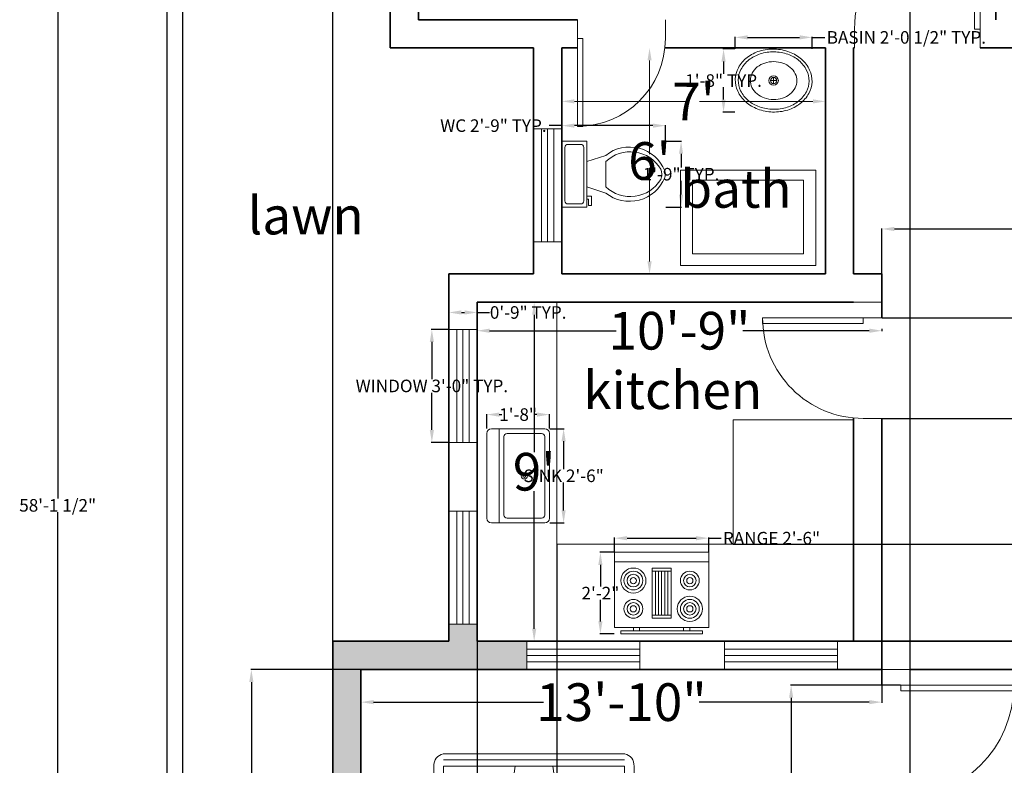
# Model space of a CAD drawing. Units: inches. Extents: x -346 to 220, y 97 to 877.
# Tile 2 of 4: x -346 to -32, y 404 to 642. Entities that reach past the tile are written whole.
import ezdxf

# ---------------------------------------------------------------- set-up
doc = ezdxf.new("R2010")
doc.units = ezdxf.units.IN
doc.header["$MEASUREMENT"] = 0
doc.layers.get('0').update_dxf_attribs({"color": 3})
for name, color, linetype, lineweight in [('A-AREA-IDEN', 130, 'Continuous', 25), ('A-EQPM', 8, 'Continuous', 18), ('A-FLOR-CABN', 8, 'Continuous', 20), ('A-FLOR-FIXT', 9, 'Continuous', 18), ('A-WALL', 7, 'Continuous', 35), ('C-PRKG-VEHI', 8, 'Continuous', 13), ('C-PROP', 94, 'Continuous', 25), ('dim', 170, 'Continuous', 13), ('door', 20, 'Continuous', 18), ('window', 230, 'Continuous', 18)]:
    doc.layers.add(name, color=color, linetype=linetype, lineweight=lineweight)
doc.layers.add('A-WALL-PATT', color=61, linetype='Continuous', lineweight=13, true_color=0xe5e878)
doc.styles.get("Standard").update_dxf_attribs({"font": 'arial.ttf'})
doc.dimstyles.get("Standard").update_dxf_attribs({"dimtxt": 4, "dimasz": 4, "dimexe": 0.18, "dimexo": 0.0625, "dimgap": 0.09, "dimtad": 0, "dimtih": 1, "dimtoh": 1, "dimdec": 0, "dimzin": 0, "dimdsep": 46, "dimlunit": 3, "dimtxsty": 'Standard', "dimcen": 0.09, "dimadec": 0, "dimazin": 0, "dimtfac": 1, "dimtdec": 0, "dimtofl": 0, "dimtmove": 0, "dimatfit": 3, "dimfxl": 1, "dimtolj": 1, "dimtzin": 0, "dimarcsym": 0})

# ---------------------------------------------------------------- blocks, each defined once
blk = doc.blocks.new('*D6')
at = {"layer": 'Defpoints', "color": 0, "transparency": 16777216}
for p in [(120.77, 575.08), (-71.23, 560.75), (120.77, 560.75)]:
    blk.add_point(p, dxfattribs=at)
at = {"layer": 'dim', "color": 0, "lineweight": -2, "transparency": 16777216}
for p, q in [((-71.23, 560.81), (-71.23, 575.26)), ((-67.23, 575.08), (15.07, 575.08)), ((116.77, 575.08), (34.48, 575.08)), ((120.77, 560.81), (120.77, 575.26))]:
    blk.add_line(p, q, dxfattribs=at)
at = {"layer": 'dim', "color": 0, "transparency": 16777216}
for points in [[(-67.23, 575.75), (-67.23, 574.41), (-71.23, 575.08)], [(116.77, 575.75), (116.77, 574.41), (120.77, 575.08)]]:
    blk.add_solid(points, dxfattribs=at)
at = {"layer": 'dim', "color": 0, "transparency": 16777216, "insert": (24.77, 575.08), "char_height": 4, "attachment_point": 5}
blk.add_mtext("\\A1;{\\H3x;16'}", dxfattribs=at)
blk = doc.blocks.new('*D8')
at = {"layer": 'Defpoints', "color": 0, "transparency": 16777216}
for p in [(-237.23, 434.75), (-71.23, 434.75), (-237.23, 424.36)]:
    blk.add_point(p, dxfattribs=at)
at = {"layer": 'dim', "color": 0, "lineweight": -2, "transparency": 16777216}
for p, q in [((-237.23, 434.68), (-237.23, 424.18)), ((-71.23, 434.68), (-71.23, 424.18)), ((-233.23, 424.36), (-179.02, 424.36)), ((-75.23, 424.36), (-129.43, 424.36))]:
    blk.add_line(p, q, dxfattribs=at)
at = {"layer": 'dim', "color": 0, "transparency": 16777216}
for points in [[(-233.23, 425.03), (-233.23, 423.7), (-237.23, 424.36)], [(-75.23, 425.03), (-75.23, 423.7), (-71.23, 424.36)]]:
    blk.add_solid(points, dxfattribs=at)
at = {"layer": 'dim', "color": 0, "transparency": 16777216, "insert": (-154.23, 424.36), "char_height": 4, "attachment_point": 5}
blk.add_mtext('\\A1;{\\H3x;13\'-10"}', dxfattribs=at)
blk = doc.blocks.new('*U13')
for p, q in [((0, 0), (0, -6)), ((36, 0), (36, -6))]:
    blk.add_line(p, q)
blk.add_lwpolyline([(0, 0), (0, 36), (1.75, 36), (1.75, 0)], close=True)
blk.add_arc((0, 0), 36, 0, 90)
blk = doc.blocks.new('*U14')
for p, q in [((0, 0), (0, 6)), ((32, 0), (32, 6))]:
    blk.add_line(p, q)
blk.add_lwpolyline([(0, 0), (0, -32), (1.75, -32), (1.75, 0)], close=True)
blk.add_arc((0, 0), 32, 270, 0)
blk = doc.blocks.new('*D15')
at = {"layer": 'Defpoints', "color": 0, "transparency": 16777216}
for p in [(-200.23, 543.36), (-71.23, 543.36), (-200.23, 542.67)]:
    blk.add_point(p, dxfattribs=at)
at = {"layer": 'dim', "color": 0, "lineweight": -2, "transparency": 16777216}
for p, q in [((-200.23, 543.29), (-200.23, 542.49)), ((-71.23, 543.29), (-71.23, 542.49)), ((-196.23, 542.67), (-155.86, 542.67)), ((-75.23, 542.67), (-115.59, 542.67))]:
    blk.add_line(p, q, dxfattribs=at)
at = {"layer": 'dim', "color": 0, "transparency": 16777216}
for points in [[(-196.23, 543.34), (-196.23, 542.01), (-200.23, 542.67)], [(-75.23, 543.34), (-75.23, 542.01), (-71.23, 542.67)]]:
    blk.add_solid(points, dxfattribs=at)
at = {"layer": 'dim', "color": 0, "transparency": 16777216, "insert": (-135.73, 542.67), "char_height": 4, "attachment_point": 5}
blk.add_mtext('\\A1;{\\H3x;10\'-9"}', dxfattribs=at)
blk = doc.blocks.new('*D16')
at = {"layer": 'Defpoints', "color": 0, "transparency": 16777216}
for p in [(-200.23, 551.75), (-200.23, 443.75), (-182.03, 443.75)]:
    blk.add_point(p, dxfattribs=at)
at = {"layer": 'dim', "color": 0, "lineweight": -2, "transparency": 16777216}
for p, q in [((-200.16, 551.75), (-181.85, 551.75)), ((-182.03, 547.75), (-182.03, 503.96)), ((-182.03, 447.75), (-182.03, 491.53)), ((-200.16, 443.75), (-181.85, 443.75))]:
    blk.add_line(p, q, dxfattribs=at)
at = {"layer": 'dim', "color": 0, "transparency": 16777216}
for points in [[(-182.69, 547.75), (-181.36, 547.75), (-182.03, 551.75)], [(-182.69, 447.75), (-181.36, 447.75), (-182.03, 443.75)]]:
    blk.add_solid(points, dxfattribs=at)
at = {"layer": 'dim', "color": 0, "transparency": 16777216, "insert": (-182.03, 497.75), "char_height": 4, "attachment_point": 5}
blk.add_mtext("\\A1;{\\H3x;9'}", dxfattribs=at)
blk = doc.blocks.new('*U17')
for p, q in [((0, 0), (0, 6)), ((28, 0), (28, 6))]:
    blk.add_line(p, q)
blk.add_lwpolyline([(0, 0), (0, -28), (1.75, -28), (1.75, 0)], close=True)
blk.add_arc((0, 0), 28, 270, 0)
blk = doc.blocks.new('*U18')
for p, q in [((0, 0), (0, -6)), ((-40, 0), (-40, -6))]:
    blk.add_line(p, q)
blk.add_lwpolyline([(0, 0), (0, 40), (-1.75, 40), (-1.75, 0)], close=True)
blk.add_arc((0, 0), 40, 90, 180)
blk = doc.blocks.new('Toilet - top')
for p, q in [((9.5, -6), (9.5, -2)), ((-10, -8.5), (-8, -8.5)), ((-10, -9.5), (-10, -8.5)), ((-8, -8.5), (-8, -8)), ((-7, -8), (-7, -9.5)), ((-4, -8), (-6, -14)), ((4, -8), (6, -14)), ((-7, -9.5), (-10, -9.5)), ((4, -14), (-4, -14))]:
    blk.add_line(p, q)
blk.add_lwpolyline([(10.5, -8), (10.5, 0), (-10.5, 0), (-10.5, -8)], close=True)
for points in [[(-9.5, -2), (-9.5, -6)], [(8.5, -1), (-8.5, -1)], [(-8.5, -7), (8.5, -7)]]:
    blk.add_lwpolyline(points)
for centre, radius, start, end in [((-8.62, -1.88), 0.884, 81.8699, 188.1301), ((8.62, -1.88), 0.884, 351.8699, 98.1301), ((-8.62, -6.12), 0.884, 171.8699, 278.1301), ((8.62, -6.12), 0.884, 261.8699, 8.1301), ((3.52, -21.58), 12.17, 141.4691, 247.9714), ((4.2, -21.82), 11.33, 136.3677, 238.9468), ((-3.52, -21.58), 12.17, 292.0284, 38.5307), ((-4.2, -21.82), 11.33, 301.053, 43.6321), ((0, -27.88), 4, 245.7318, 294.2682), ((0, -29), 4, 254.8605, 285.1395)]:
    blk.add_arc(centre, radius, start, end)
blk = doc.blocks.new('Range-Oven - 30 in top')
for p, q in [((0, -3), (30, -3)), ((12, -6), (18, -6)), ((13, -20), (13, -6)), ((14, -6), (14, -20)), ((15, -20), (15, -6)), ((16, -6), (16, -20)), ((17, -20), (17, -6)), ((18, -20), (12, -20)), ((6, -24), (6, -25)), ((8, -25), (8, -24)), ((22, -25), (22, -24)), ((24, -24), (24, -25))]:
    blk.add_line(p, q)
for points in [[(0, -24), (0, 0), (30, 0), (30, -24)], [(12, -21), (12, -5), (18, -5), (18, -21)], [(2, -26), (2, -25), (28, -25), (28, -26)]]:
    blk.add_lwpolyline(points, close=True)
for centre, radius in [((6, -9), 4), ((6, -9), 3), ((24, -9), 3), ((6, -9), 2), ((6, -9), 1), ((24, -9), 2), ((24, -9), 1), ((6, -18), 3), ((24, -18), 4), ((24, -18), 3), ((6, -18), 2), ((6, -18), 1), ((24, -18), 2), ((24, -18), 1)]:
    blk.add_circle(centre, radius)
blk = doc.blocks.new('Sink-single - 30 in top')
blk.add_line((-15, -3.999996), (15, -3.999996))
for points in [[(-13.5, 0), (13.5, 0)], [(-15, -18.499996), (-15, -1.5)], [(15, -1.5), (15, -18.499996)], [(-12.5, -5.499996), (12.5, -5.499996)], [(-13.5, -17.499996), (-13.5, -6.499996)], [(13.5, -6.499996), (13.5, -17.499996)], [(12.5, -18.499996), (-12.5, -18.499996)], [(13.5, -19.999996), (-13.5, -19.999996)]]:
    blk.add_lwpolyline(points)
for radius in [1, 0.5]:
    blk.add_circle((0, -11.999996), radius)
for centre, radius, start, end in [((-13.5, -1.5), 1.5, 90, 180), ((13.5, -1.5), 1.5, 0, 90), ((-12.5, -6.499996), 1, 90, 180), ((12.5, -6.499996), 1, 0, 90), ((-13.5, -18.499996), 1.5, 180, 270), ((-12.5, -17.499996), 1, 180, 270), ((12.5, -17.499996), 1, 270, 0), ((13.5, -18.499996), 1.5, 270, 0)]:
    blk.add_arc(centre, radius, start, end)
blk = doc.blocks.new('Sink - Oval top')
for p, q in [((-1, 0), (1, 0)), ((0, 1), (0, -1))]:
    blk.add_line(p, q)
for points in [[(-12.23, 0.39, 0.117634), (-11.46, -3.36, 0.104469), (-8.88, -6.8, 0.090016), (-5.08, -9.07, 0.08192), (-0.32, -10.02, 0.08192), (4.49, -9.38, 0.090016), (8.42, -7.36, 0.104469), (11.22, -4.09, 0.117634), (12.23, -0.39, 0.117634), (11.46, 3.36, 0.104469), (8.88, 6.8, 0.090016), (5.08, 9.07, 0.08192), (0.32, 10.02, 0.08192), (-4.49, 9.38, 0.090016), (-8.42, 7.36, 0.104469), (-11.22, 4.09, 0.117634)], [(-11.29, 0.16, 0.118622), (-10.52, -3.25, 0.104678), (-8.07, -6.36, 0.089562), (-4.54, -8.37, 0.081185), (-0.13, -9.15, 0.081185), (4.3, -8.49, 0.089562), (7.89, -6.58, 0.104678), (10.42, -3.55, 0.118622), (11.29, -0.16, 0.118622), (10.52, 3.25, 0.104678), (8.07, 6.36, 0.089562), (4.54, 8.37, 0.081185), (0.13, 9.15, 0.081185), (-4.3, 8.49, 0.089562), (-7.89, 6.58, 0.104678), (-10.42, 3.55, 0.118622)], [(-7.42, 0.08, 0.118283), (-6.91, -2.17, 0.104607), (-5.29, -4.21, 0.089718), (-2.97, -5.53, 0.081436), (-0.07, -6.04, 0.081436), (2.84, -5.59, 0.089718), (5.2, -4.33, 0.104607), (6.86, -2.32, 0.118283), (7.42, -0.08, 0.118283), (6.91, 2.17, 0.104607), (5.29, 4.21, 0.089718), (2.97, 5.53, 0.081436), (0.07, 6.04, 0.081436), (-2.84, 5.59, 0.089718), (-5.2, 4.33, 0.104607), (-6.86, 2.32, 0.118283)]]:
    blk.add_lwpolyline(points, format="xyb", close=True)
for radius in [1.5, 1]:
    blk.add_circle((0, 0), radius)
blk = doc.blocks.new('*U27')
for p, q in [((5.44, 42.31), (12.12, 42.31)), ((189.69, 42.31), (183.01, 42.31)), ((0.1, -0.41), (0.1, 38.35)), ((2.77, -0.41), (2.77, 38.31)), ((5.44, -0.41), (5.44, 38.24)), ((5.45, 38.31), (16.12, 38.31)), ((16.12, 38.31), (180.34, 38.31)), ((61.52, -0.41), (61.52, 38.31)), ((61.52, 38.31), (77.54, 27.62)), ((64.19, 38.31), (76.2, 30.29)), ((76.2, 30.29), (76.2, 38.31)), ((78.87, 38.31), (78.87, 28.96)), ((106.91, 28.96), (106.91, 38.31)), ((109.58, 27.62), (109.58, 38.31)), ((112.25, 38.31), (112.25, 28.96)), ((140.29, 28.96), (140.29, 38.31)), ((141.62, 27.62), (149.64, 38.31)), ((149.64, -0.41), (149.64, 38.31)), ((189.69, 38.31), (179.01, 38.31)), ((189.69, -0.41), (189.69, 38.24)), ((192.36, -0.41), (192.36, 38.31)), ((195.03, -0.41), (195.03, 38.35)), ((77.54, 27.62), (141.62, 27.62)), ((77.54, -0.41), (77.54, 27.62)), ((78.87, 28.96), (106.91, 28.96)), ((112.25, 28.96), (140.29, 28.96)), ((141.62, -0.41), (141.62, 27.62)), ((5.44, 7.6), (61.52, 15.61)), ((0.1, -0.42), (0.1, -39.18)), ((2.77, -0.41), (2.77, -39.13)), ((5.44, -0.42), (5.44, -39.07)), ((61.52, -0.41), (61.52, -39.13)), ((77.54, -0.41), (77.54, -28.45)), ((141.62, -0.41), (141.62, -28.45)), ((149.64, -0.41), (149.64, -39.13)), ((189.69, -0.42), (189.69, -39.07)), ((192.36, -0.41), (192.36, -39.13)), ((195.03, -0.42), (195.03, -39.18)), ((5.44, -8.42), (61.52, -16.43)), ((61.52, -39.13), (77.54, -28.45)), ((77.54, -28.45), (141.62, -28.45)), ((109.58, -28.45), (109.58, -39.13)), ((141.62, -28.45), (149.64, -39.13)), ((64.19, -39.13), (76.2, -31.12)), ((76.2, -31.12), (76.2, -39.13)), ((78.87, -39.13), (78.87, -29.79)), ((78.87, -29.79), (106.91, -29.79)), ((106.91, -29.79), (106.91, -39.13)), ((112.25, -29.79), (140.29, -29.79)), ((112.25, -39.13), (112.25, -29.79)), ((140.29, -29.79), (140.29, -39.13)), ((5.45, -39.13), (16.12, -39.13)), ((16.12, -39.13), (180.34, -39.13)), ((189.69, -39.13), (179.01, -39.13)), ((5.44, -43.14), (12.12, -43.14)), ((189.69, -43.14), (183.01, -43.14))]:
    blk.add_line(p, q)
for centre, radius, start, end in [((5.06, 37.26), 5.06, 85.6455, 168.0943), ((11.45, 37.64), 4.72, 8.1301, 81.87), ((183.68, 37.64), 4.72, 98.13, 171.8699), ((190.07, 37.26), 5.06, 11.9057, 94.3545), ((5.06, -38.09), 5.06, 191.9057, 274.3545), ((11.45, -38.46), 4.72, 278.13, 351.8699), ((183.68, -38.46), 4.72, 188.1301, 261.87), ((190.07, -38.09), 5.06, 265.6455, 348.0943)]:
    blk.add_arc(centre, radius, start, end)
blk = doc.blocks.new('WIN-36x9-PLAN')
for p, q in [((2.5, 36), (2.5, 0)), ((4.5, 36), (4.5, 0)), ((6.5, 36), (6.5, 0))]:
    blk.add_line(p, q)
blk.add_lwpolyline([(0, 36), (9, 36), (9, 0), (0, 0)], close=True)
blk = doc.blocks.new('*D30')
at = {"layer": 'Defpoints', "color": 0, "transparency": 16777216}
for p in [(-214.63, 543.09), (-209.23, 543.09), (-209.23, 507.09)]:
    blk.add_point(p, dxfattribs=at)
at = {"layer": 'dim', "color": 0, "lineweight": -2, "transparency": 16777216}
for p, q in [((-209.3, 543.09), (-214.81, 543.09)), ((-214.63, 539.09), (-214.63, 527.25)), ((-214.63, 511.09), (-214.63, 522.93)), ((-209.3, 507.09), (-214.81, 507.09))]:
    blk.add_line(p, q, dxfattribs=at)
at = {"layer": 'dim', "color": 0, "transparency": 16777216}
for points in [[(-215.3, 539.09), (-213.97, 539.09), (-214.63, 543.09)], [(-215.3, 511.09), (-213.97, 511.09), (-214.63, 507.09)]]:
    blk.add_solid(points, dxfattribs=at)
at = {"layer": 'dim', "color": 0, "transparency": 16777216, "insert": (-214.63, 525.09), "char_height": 4, "attachment_point": 5}
blk.add_mtext('\\A1;WINDOW 3\'-0" TYP.', dxfattribs=at)
blk = doc.blocks.new('*D31')
at = {"layer": 'Defpoints', "color": 0, "transparency": 16777216}
for p in [(-200.23, 548.49), (-209.23, 543.09), (-200.23, 543.09)]:
    blk.add_point(p, dxfattribs=at)
at = {"layer": 'dim', "color": 0, "lineweight": -2, "transparency": 16777216}
for p, q in [((-209.23, 543.15), (-209.23, 548.67)), ((-205.23, 548.49), (-204.23, 548.49)), ((-200.23, 543.15), (-200.23, 548.67)), ((-200.23, 548.49), (-196.23, 548.49))]:
    blk.add_line(p, q, dxfattribs=at)
at = {"layer": 'dim', "color": 0, "transparency": 16777216}
for points in [[(-205.23, 549.15), (-205.23, 547.82), (-209.23, 548.49)], [(-204.23, 549.15), (-204.23, 547.82), (-200.23, 548.49)]]:
    blk.add_solid(points, dxfattribs=at)
at = {"layer": 'dim', "color": 0, "transparency": 16777216, "insert": (-183.95, 548.49), "char_height": 4, "attachment_point": 5}
blk.add_mtext('\\A1;0\'-9" TYP.', dxfattribs=at)
blk = doc.blocks.new('*D36')
at = {"layer": 'Defpoints', "color": 0, "transparency": 16777216}
for p in [(-173.23, 608), (-173.23, 603.04), (-140.18, 603.04)]:
    blk.add_point(p, dxfattribs=at)
at = {"layer": 'dim', "color": 0, "lineweight": -2, "transparency": 16777216}
for p, q in [((-173.23, 608), (-177.23, 608)), ((-173.23, 603.11), (-173.23, 608.18)), ((-144.18, 608), (-169.23, 608)), ((-140.18, 603.11), (-140.18, 608.18))]:
    blk.add_line(p, q, dxfattribs=at)
at = {"layer": 'dim', "color": 0, "transparency": 16777216}
for points in [[(-169.23, 608.67), (-169.23, 607.33), (-173.23, 608)], [(-144.18, 608.67), (-144.18, 607.33), (-140.18, 608)]]:
    blk.add_solid(points, dxfattribs=at)
at = {"layer": 'dim', "color": 0, "transparency": 16777216, "insert": (-195.02, 608), "char_height": 4, "attachment_point": 5}
blk.add_mtext('\\A1;WC 2\'-9" TYP.', dxfattribs=at)
blk = doc.blocks.new('*D37')
at = {"layer": 'Defpoints', "color": 0, "transparency": 16777216}
for p in [(-140.18, 603.04), (-135.22, 603.04), (-140.18, 582.04)]:
    blk.add_point(p, dxfattribs=at)
at = {"layer": 'dim', "color": 0, "lineweight": -2, "transparency": 16777216}
for p, q in [((-140.12, 603.04), (-135.04, 603.04)), ((-135.22, 599.04), (-135.22, 594.68)), ((-135.22, 586.04), (-135.22, 590.41)), ((-140.12, 582.04), (-135.04, 582.04))]:
    blk.add_line(p, q, dxfattribs=at)
at = {"layer": 'dim', "color": 0, "transparency": 16777216}
for points in [[(-135.89, 599.04), (-134.56, 599.04), (-135.22, 603.04)], [(-135.89, 586.04), (-134.56, 586.04), (-135.22, 582.04)]]:
    blk.add_solid(points, dxfattribs=at)
at = {"layer": 'dim', "color": 0, "transparency": 16777216, "insert": (-135.22, 592.54), "char_height": 4, "attachment_point": 5}
blk.add_mtext('\\A1;1\'-9" TYP.', dxfattribs=at)
blk = doc.blocks.new('*D40')
at = {"layer": 'Defpoints', "color": 0, "transparency": 16777216}
for p in [(-93.45, 636.11), (-118, 632.43), (-93.45, 632.43)]:
    blk.add_point(p, dxfattribs=at)
at = {"layer": 'dim', "color": 0, "lineweight": -2, "transparency": 16777216}
for p, q in [((-118, 632.49), (-118, 636.29)), ((-114, 636.11), (-97.45, 636.11)), ((-93.45, 632.49), (-93.45, 636.29)), ((-93.45, 636.11), (-89.45, 636.11))]:
    blk.add_line(p, q, dxfattribs=at)
at = {"layer": 'dim', "color": 0, "transparency": 16777216}
for points in [[(-114, 636.78), (-114, 635.45), (-118, 636.11)], [(-97.45, 636.78), (-97.45, 635.45), (-93.45, 636.11)]]:
    blk.add_solid(points, dxfattribs=at)
at = {"layer": 'dim', "color": 0, "transparency": 16777216, "insert": (-63.43, 636.11), "char_height": 4, "attachment_point": 5}
blk.add_mtext('\\A1;BASIN 2\'-0 1/2" TYP.', dxfattribs=at)
blk = doc.blocks.new('*D41')
at = {"layer": 'Defpoints', "color": 0, "transparency": 16777216}
for p in [(-121.68, 632.43), (-118, 632.43), (-118, 612.3)]:
    blk.add_point(p, dxfattribs=at)
at = {"layer": 'dim', "color": 0, "lineweight": -2, "transparency": 16777216}
for p, q in [((-118.06, 632.43), (-121.86, 632.43)), ((-121.68, 628.43), (-121.68, 624.5)), ((-121.68, 616.3), (-121.68, 620.23)), ((-118.06, 612.3), (-121.86, 612.3))]:
    blk.add_line(p, q, dxfattribs=at)
at = {"layer": 'dim', "color": 0, "transparency": 16777216}
for points in [[(-122.35, 628.43), (-121.02, 628.43), (-121.68, 632.43)], [(-122.35, 616.3), (-121.02, 616.3), (-121.68, 612.3)]]:
    blk.add_solid(points, dxfattribs=at)
at = {"layer": 'dim', "color": 0, "transparency": 16777216, "insert": (-121.68, 622.36), "char_height": 4, "attachment_point": 5}
blk.add_mtext('\\A1;1\'-8" TYP.', dxfattribs=at)
blk = doc.blocks.new('*D44')
at = {"layer": 'Defpoints', "color": 0, "transparency": 16777216}
for p in [(-126.42, 476.59), (-156.42, 472.09), (-126.42, 472.09)]:
    blk.add_point(p, dxfattribs=at)
at = {"layer": 'dim', "color": 0, "lineweight": -2, "transparency": 16777216}
for p, q in [((-156.42, 472.15), (-156.42, 476.77)), ((-152.42, 476.59), (-130.42, 476.59)), ((-126.42, 472.15), (-126.42, 476.77)), ((-126.42, 476.59), (-122.42, 476.59))]:
    blk.add_line(p, q, dxfattribs=at)
at = {"layer": 'dim', "color": 0, "transparency": 16777216}
for points in [[(-152.42, 477.25), (-152.42, 475.92), (-156.42, 476.59)], [(-130.42, 477.25), (-130.42, 475.92), (-126.42, 476.59)]]:
    blk.add_solid(points, dxfattribs=at)
at = {"layer": 'dim', "color": 0, "transparency": 16777216, "insert": (-106.41, 476.59), "char_height": 4, "attachment_point": 5}
blk.add_mtext('\\A1;RANGE 2\'-6"', dxfattribs=at)
blk = doc.blocks.new('*D45')
at = {"layer": 'Defpoints', "color": 0, "transparency": 16777216}
for p in [(-160.92, 472.09), (-156.42, 472.09), (-156.42, 446.09)]:
    blk.add_point(p, dxfattribs=at)
at = {"layer": 'dim', "color": 0, "lineweight": -2, "transparency": 16777216}
for p, q in [((-156.49, 472.09), (-161.1, 472.09)), ((-160.92, 468.09), (-160.92, 461.18)), ((-160.92, 450.09), (-160.92, 456.99)), ((-156.49, 446.09), (-161.1, 446.09))]:
    blk.add_line(p, q, dxfattribs=at)
at = {"layer": 'dim', "color": 0, "transparency": 16777216}
for points in [[(-161.59, 468.09), (-160.26, 468.09), (-160.92, 472.09)], [(-161.59, 450.09), (-160.26, 450.09), (-160.92, 446.09)]]:
    blk.add_solid(points, dxfattribs=at)
at = {"layer": 'dim', "color": 0, "transparency": 16777216, "insert": (-160.92, 459.09), "char_height": 4, "attachment_point": 5}
blk.add_mtext('\\A1;2\'-2"', dxfattribs=at)
blk = doc.blocks.new('*D46')
at = {"layer": 'Defpoints', "color": 0, "transparency": 16777216}
for p in [(-177.15, 511.46), (-172.65, 511.46), (-177.15, 481.46)]:
    blk.add_point(p, dxfattribs=at)
at = {"layer": 'dim', "color": 0, "lineweight": -2, "transparency": 16777216}
for p, q in [((-177.09, 511.46), (-172.47, 511.46)), ((-172.65, 507.46), (-172.65, 498.62)), ((-172.65, 485.46), (-172.65, 494.3)), ((-177.09, 481.46), (-172.47, 481.46))]:
    blk.add_line(p, q, dxfattribs=at)
at = {"layer": 'dim', "color": 0, "transparency": 16777216}
for points in [[(-173.32, 507.46), (-171.99, 507.46), (-172.65, 511.46)], [(-173.32, 485.46), (-171.99, 485.46), (-172.65, 481.46)]]:
    blk.add_solid(points, dxfattribs=at)
at = {"layer": 'dim', "color": 0, "transparency": 16777216, "insert": (-172.65, 496.46), "char_height": 4, "attachment_point": 5}
blk.add_mtext('\\A1;SINK 2\'-6"', dxfattribs=at)
blk = doc.blocks.new('*D47')
at = {"layer": 'Defpoints', "color": 0, "transparency": 16777216}
for p in [(-197.15, 515.96), (-197.15, 511.46), (-177.15, 511.46)]:
    blk.add_point(p, dxfattribs=at)
at = {"layer": 'dim', "color": 0, "lineweight": -2, "transparency": 16777216}
for p, q in [((-197.15, 511.52), (-197.15, 516.14)), ((-193.15, 515.96), (-192.37, 515.96)), ((-181.15, 515.96), (-181.94, 515.96)), ((-177.15, 511.52), (-177.15, 516.14))]:
    blk.add_line(p, q, dxfattribs=at)
at = {"layer": 'dim', "color": 0, "transparency": 16777216}
for points in [[(-193.15, 516.63), (-193.15, 515.29), (-197.15, 515.96)], [(-181.15, 516.63), (-181.15, 515.29), (-177.15, 515.96)]]:
    blk.add_solid(points, dxfattribs=at)
at = {"layer": 'dim', "color": 0, "transparency": 16777216, "insert": (-187.15, 515.96), "char_height": 4, "attachment_point": 5}
blk.add_mtext('\\A1;1\'-8"', dxfattribs=at)
blk = doc.blocks.new('*D49')
at = {"layer": 'Defpoints', "color": 0, "transparency": 16777216}
for p in [(-333.87, 835.75), (-298.95, 835.75), (-298.95, 138.35)]:
    blk.add_point(p, dxfattribs=at)
at = {"layer": 'dim', "color": 0, "lineweight": -2, "transparency": 16777216}
for p, q in [((-299.01, 835.75), (-334.05, 835.75)), ((-333.87, 831.75), (-333.87, 489.21)), ((-333.87, 142.35), (-333.87, 484.89)), ((-299.01, 138.35), (-334.05, 138.35))]:
    blk.add_line(p, q, dxfattribs=at)
at = {"layer": 'dim', "color": 0, "transparency": 16777216}
for points in [[(-334.54, 831.75), (-333.21, 831.75), (-333.87, 835.75)], [(-334.54, 142.35), (-333.21, 142.35), (-333.87, 138.35)]]:
    blk.add_solid(points, dxfattribs=at)
at = {"layer": 'dim', "color": 0, "transparency": 16777216, "insert": (-333.87, 487.05), "char_height": 4, "attachment_point": 5}
blk.add_mtext('\\A1;58\'-1 1/2"', dxfattribs=at)
blk = doc.blocks.new('*D52')
at = {"layer": 'Defpoints', "color": 0, "transparency": 16777216}
for p in [(-246.23, 870.67), (-246.23, 242.75), (-293.95, 143.35)]:
    blk.add_point(p, dxfattribs=at)
at = {"layer": 'dim', "color": 0, "lineweight": -2, "transparency": 16777216}
for p, q in [((-293.95, 143.41), (-293.95, 870.85)), ((-289.95, 870.67), (-281.71, 870.67)), ((-250.23, 870.67), (-258.47, 870.67)), ((-246.23, 242.81), (-246.23, 870.85))]:
    blk.add_line(p, q, dxfattribs=at)
at = {"layer": 'dim', "color": 0, "transparency": 16777216}
for points in [[(-289.95, 871.34), (-289.95, 870), (-293.95, 870.67)], [(-250.23, 871.34), (-250.23, 870), (-246.23, 870.67)]]:
    blk.add_solid(points, dxfattribs=at)
at = {"layer": 'dim', "color": 0, "transparency": 16777216, "insert": (-270.09, 870.67), "char_height": 4, "attachment_point": 5}
blk.add_mtext('\\A1;3\'-11 1/2"', dxfattribs=at)
blk = doc.blocks.new('*D58')
at = {"layer": 'Defpoints', "color": 0, "transparency": 16777216}
for p in [(3.77, 870.67), (3.77, 341.75), (-62.23, 331.75)]:
    blk.add_point(p, dxfattribs=at)
at = {"layer": 'dim', "color": 0, "lineweight": -2, "transparency": 16777216}
for p, q in [((-62.23, 331.81), (-62.23, 870.85)), ((-58.23, 870.67), (-34.63, 870.67)), ((-0.23, 870.67), (-23.82, 870.67)), ((3.77, 341.81), (3.77, 870.85))]:
    blk.add_line(p, q, dxfattribs=at)
at = {"layer": 'dim', "color": 0, "transparency": 16777216}
for points in [[(-58.23, 871.34), (-58.23, 870), (-62.23, 870.67)], [(-0.23, 871.34), (-0.23, 870), (3.77, 870.67)]]:
    blk.add_solid(points, dxfattribs=at)
at = {"layer": 'dim', "color": 0, "transparency": 16777216, "insert": (-29.23, 870.67), "char_height": 4, "attachment_point": 5}
blk.add_mtext('\\A1;5\'-6"', dxfattribs=at)
blk = doc.blocks.new('*D59')
at = {"layer": 'Defpoints', "color": 0, "transparency": 16777216}
for p in [(-272.15, 434.75), (-237.23, 434.75), (-237.23, 251.75)]:
    blk.add_point(p, dxfattribs=at)
at = {"layer": 'dim', "color": 0, "lineweight": -2, "transparency": 16777216}
for p, q in [((-237.29, 434.75), (-272.33, 434.75)), ((-272.15, 430.75), (-272.15, 345.38)), ((-272.15, 255.75), (-272.15, 341.11)), ((-237.29, 251.75), (-272.33, 251.75))]:
    blk.add_line(p, q, dxfattribs=at)
at = {"layer": 'dim', "color": 0, "transparency": 16777216}
for points in [[(-272.82, 430.75), (-271.48, 430.75), (-272.15, 434.75)], [(-272.82, 255.75), (-271.48, 255.75), (-272.15, 251.75)]]:
    blk.add_solid(points, dxfattribs=at)
at = {"layer": 'dim', "color": 0, "transparency": 16777216, "insert": (-272.15, 343.25), "char_height": 4, "attachment_point": 5}
blk.add_mtext('\\A1;15\'-3"', dxfattribs=at)
blk = doc.blocks.new('*D61')
at = {"layer": 'Defpoints', "color": 0, "transparency": 16777216}
for p in [(-100.15, 429.75), (-65.23, 429.75), (-65.23, 357.75)]:
    blk.add_point(p, dxfattribs=at)
at = {"layer": 'dim', "color": 0, "lineweight": -2, "transparency": 16777216}
for p, q in [((-65.29, 429.75), (-100.33, 429.75)), ((-100.15, 425.75), (-100.15, 395.88)), ((-100.15, 361.75), (-100.15, 391.61)), ((-65.29, 357.75), (-100.33, 357.75))]:
    blk.add_line(p, q, dxfattribs=at)
at = {"layer": 'dim', "color": 0, "transparency": 16777216}
for points in [[(-100.82, 425.75), (-99.48, 425.75), (-100.15, 429.75)], [(-100.82, 361.75), (-99.48, 361.75), (-100.15, 357.75)]]:
    blk.add_solid(points, dxfattribs=at)
at = {"layer": 'dim', "color": 0, "transparency": 16777216, "insert": (-100.15, 393.75), "char_height": 4, "attachment_point": 5}
blk.add_mtext('\\A1;6\'-0"', dxfattribs=at)
blk = doc.blocks.new('*D63')
at = {"layer": 'Defpoints', "color": 0, "transparency": 16777216}
for p in [(-71.23, 546.75), (212, 546.75), (-71.23, 514.75)]:
    blk.add_point(p, dxfattribs=at)
at = {"layer": 'dim', "color": 0, "lineweight": -2, "transparency": 16777216}
for p, q in [((-71.16, 546.75), (212.18, 546.75)), ((212, 542.75), (212, 532.88)), ((212, 518.75), (212, 528.61)), ((-71.16, 514.75), (212.18, 514.75))]:
    blk.add_line(p, q, dxfattribs=at)
at = {"layer": 'dim', "color": 0, "transparency": 16777216}
for points in [[(211.33, 542.75), (212.66, 542.75), (212, 546.75)], [(211.33, 518.75), (212.66, 518.75), (212, 514.75)]]:
    blk.add_solid(points, dxfattribs=at)
at = {"layer": 'dim', "color": 0, "transparency": 16777216, "insert": (212, 530.75), "char_height": 4, "attachment_point": 5}
blk.add_mtext('\\A1;2\'-8"', dxfattribs=at)
blk = doc.blocks.new('*D71')
at = {"layer": 'Defpoints', "color": 0, "transparency": 16777216}
for p in [(-174.82, 474.69), (-200.23, 443.75), (-174.82, 103.43)]:
    blk.add_point(p, dxfattribs=at)
at = {"layer": 'dim', "color": 0, "lineweight": -2, "transparency": 16777216}
for p, q in [((-174.82, 474.63), (-174.82, 103.25)), ((-200.23, 443.68), (-200.23, 103.25)), ((-204.23, 103.43), (-208.23, 103.43)), ((-170.82, 103.43), (-166.82, 103.43))]:
    blk.add_line(p, q, dxfattribs=at)
at = {"layer": 'dim', "color": 0, "transparency": 16777216}
for points in [[(-204.23, 104.09), (-204.23, 102.76), (-200.23, 103.43)], [(-170.82, 104.09), (-170.82, 102.76), (-174.82, 103.43)]]:
    blk.add_solid(points, dxfattribs=at)
at = {"layer": 'dim', "color": 0, "transparency": 16777216, "insert": (-187.52, 103.43), "char_height": 4, "attachment_point": 5}
blk.add_mtext('\\A1;2\'-1 1/2"', dxfattribs=at)
blk = doc.blocks.new('*D72')
at = {"layer": 'Defpoints', "color": 0, "transparency": 16777216}
for p in [(-118.63, 474.69), (212, 474.69), (-80.23, 443.75)]:
    blk.add_point(p, dxfattribs=at)
at = {"layer": 'dim', "color": 0, "lineweight": -2, "transparency": 16777216}
for p, q in [((-118.57, 474.69), (212.18, 474.69)), ((212, 470.69), (212, 461.32)), ((212, 447.75), (212, 457.12)), ((-80.16, 443.75), (212.18, 443.75))]:
    blk.add_line(p, q, dxfattribs=at)
at = {"layer": 'dim', "color": 0, "transparency": 16777216}
for points in [[(211.33, 470.69), (212.66, 470.69), (212, 474.69)], [(211.33, 447.75), (212.66, 447.75), (212, 443.75)]]:
    blk.add_solid(points, dxfattribs=at)
at = {"layer": 'dim', "color": 0, "transparency": 16777216, "insert": (212, 459.22), "char_height": 4, "attachment_point": 5}
blk.add_mtext('\\A1;2\'-7"', dxfattribs=at)

msp = doc.modelspace()

# ---------------------------------------------------------------- hatches: boundary and pattern name
at = {"layer": 'A-WALL-PATT'}
h = msp.add_hatch(color=256, dxfattribs=at)
h.dxf.hatch_style = 1
h.paths.add_polyline_path([(168.07, 251.75), (33.77, 251.75), (12.77, 251.75), (12.77, 350.86, -0.01877), (9.77, 350.75), (3.77, 350.75), (3.77, 251.75), (-62.23, 251.75), (-62.23, 357.75), (-65.23, 357.75), (-71.23, 357.75), (-71.23, 242.75), (168.07, 242.75)])
h.paths.add_polyline_path([(-71.23, 251.75), (-154.23, 251.75), (-154.23, 242.75), (-71.23, 242.75)])
h.paths.add_polyline_path([(-224.48, 251.75), (-237.23, 251.75), (-237.23, 434.75), (-184.39, 434.75), (-184.39, 443.75), (-200.23, 443.75), (-200.23, 449.16), (-209.23, 449.16), (-209.23, 443.75), (-246.23, 443.75), (-246.23, 242.75), (-224.48, 242.75)])

# ---------------------------------------------------------------- linework, layer by layer
at = {"layer": 'A-FLOR-CABN'}
for p, q in [((-174.82, 474.69), (-174.82, 551.75)), ((-80.23, 514.25), (-118.63, 514.25)), ((-118.63, 514.25), (-118.63, 474.69)), ((-118.63, 474.69), (-174.82, 474.69))]:
    msp.add_line(p, q, dxfattribs=at)
at = {"layer": 'A-FLOR-FIXT'}
for points in [[(-135.44, 593.85), (-92.26, 593.85), (-92.26, 563.46), (-135.44, 563.46)], [(-131.55, 590.63), (-96.21, 590.63), (-96.21, 567.17), (-131.55, 567.17)]]:
    msp.add_lwpolyline(points, close=True, dxfattribs=at)
at = {"layer": 'A-WALL'}
for p, q in [((-227.93, 632.75), (-227.93, 794.75)), ((-218.93, 641.75), (-218.93, 785.75)), ((-34.93, 785.75), (-34.93, 641.75)), ((-168.23, 641.75), (-218.93, 641.75)), ((-182.23, 632.75), (-227.93, 632.75)), ((-182.23, 560.75), (-182.23, 632.75)), ((-173.23, 632.75), (-168.23, 632.75)), ((-173.23, 560.75), (-173.23, 632.75)), ((-168.23, 632.75), (-173.23, 632.75)), ((-89.23, 632.75), (-140.39, 632.75)), ((-140.39, 632.75), (-89.23, 632.75)), ((-89.23, 632.75), (-89.23, 560.75)), ((-80.23, 632.75), (-80.23, 560.75)), ((-79.93, 632.75), (-80.23, 632.75)), ((-25.93, 632.75), (-39.93, 632.75)), ((-182.23, 560.75), (-209.23, 560.75)), ((-209.23, 560.75), (-209.23, 443.75)), ((-89.23, 560.75), (-173.23, 560.75)), ((-71.23, 560.75), (-80.23, 560.75)), ((-71.23, 546.75), (-71.23, 560.75)), ((-80.23, 551.75), (-200.23, 551.75)), ((-200.23, 551.75), (-200.23, 443.75)), ((-80.23, 551.75), (-182.23, 551.75)), ((-80.23, 443.75), (-80.23, 514.89)), ((-71.23, 443.75), (-71.23, 514.75)), ((-246.23, 443.75), (-246.23, 242.75)), ((-209.23, 443.75), (-246.23, 443.75)), ((-200.23, 443.75), (-80.23, 443.75)), ((-62.23, 443.75), (-200.23, 443.75)), ((-71.23, 443.75), (12.77, 443.75)), ((-71.23, 429.75), (-71.23, 443.75)), ((-71.23, 434.75), (-237.23, 434.75)), ((-237.23, 434.75), (-237.23, 251.75)), ((-209.23, 434.75), (-71.23, 434.75)), ((-71.23, 429.75), (-71.23, 434.75)), ((-62.23, 434.75), (3.77, 434.75))]:
    msp.add_line(p, q, dxfattribs=at)
at = {"layer": 'C-PROP'}
for p, q in [((-298.95, 138.35), (-298.95, 835.75)), ((-293.95, 143.35), (-293.95, 830.75))]:
    msp.add_line(p, q, dxfattribs=at)
at = {"layer": 'dim'}
for p, q in [((-173.23, 632.68), (-173.23, 615.55)), ((-131.29, 632.75), (-140.39, 632.75)), ((-89.23, 632.68), (-89.23, 615.55)), ((-145.26, 628.75), (-145.26, 598.88)), ((-169.23, 615.73), (-133.14, 615.73)), ((-93.23, 615.73), (-129.31, 615.73)), ((-145.26, 564.75), (-145.26, 594.61)), ((-131.29, 560.75), (-145.44, 560.75))]:
    msp.add_line(p, q, dxfattribs=at)
for points in [[(-145.93, 628.75), (-144.6, 628.75), (-145.26, 632.75)], [(-169.23, 616.39), (-169.23, 615.06), (-173.23, 615.73)], [(-93.23, 616.39), (-93.23, 615.06), (-89.23, 615.73)], [(-145.93, 564.75), (-144.6, 564.75), (-145.26, 560.75)]]:
    msp.add_solid(points, dxfattribs=at)
at = {"layer": 'door'}
for p, q in [((-168.23, 632.68), (-168.23, 641.75)), ((-39.93, 641.75), (-39.93, 632.75)), ((-173.23, 632.68), (-173.23, 632.75)), ((-80.23, 551.75), (-71.23, 551.75)), ((-80.23, 546.75), (-71.23, 546.75)), ((-71.23, 434.75), (-62.23, 434.75)), ((-71.23, 429.75), (-62.23, 429.75))]:
    msp.add_line(p, q, dxfattribs=at)
at = {"layer": 'window'}
for p, q in [((-206.73, 485.16), (-206.73, 449.16)), ((-204.73, 485.16), (-204.73, 449.16)), ((-202.73, 485.16), (-202.73, 449.16)), ((-148.39, 441.25), (-184.39, 441.25)), ((-148.39, 439.25), (-184.39, 439.25)), ((-148.39, 437.25), (-184.39, 437.25))]:
    msp.add_line(p, q, dxfattribs=at)
for points in [[(-209.23, 485.16), (-200.23, 485.16), (-200.23, 449.16), (-209.23, 449.16)], [(-148.39, 443.75), (-148.39, 434.75), (-184.39, 434.75), (-184.39, 443.75)]]:
    msp.add_lwpolyline(points, close=True, dxfattribs=at)

# ---------------------------------------------------------------- block references
at = {"layer": 'A-EQPM'}
msp.add_blockref('Range-Oven - 30 in top', (-156.42, 472.09), dxfattribs=at)
at = {"layer": 'A-FLOR-FIXT'}
msp.add_blockref('Sink - Oval top', (-105.72, 622.36), dxfattribs=at)
at = {"layer": 'A-FLOR-FIXT', "rotation": 90}
for name, p in [('Toilet - top', (-173.23, 592.54)), ('Sink-single - 30 in top', (-197.15, 496.46))]:
    msp.add_blockref(name, p, dxfattribs=at)
at = {"layer": 'C-PRKG-VEHI', "xscale": 0.7461287105312193, "yscale": 0.7461287105312193, "zscale": 0.7461287105312193, "rotation": 270}
msp.add_blockref('*U27', (-181.78, 408.01), dxfattribs=at)
at = {"layer": 'door'}
for name, p in [('*U18', (-39.93, 638.75)), ('*U17', (-168.23, 635.75))]:
    msp.add_blockref(name, p, dxfattribs=at)
at = {"layer": 'door', "rotation": 270}
for name, p in [('*U14', (-77.23, 546.75)), ('*U13', (-65.23, 429.75))]:
    msp.add_blockref(name, p, dxfattribs=at)
at = {"layer": 'window'}
for p in [(-182.24, 570.94), (-209.23, 507.09)]:
    msp.add_blockref('WIN-36x9-PLAN', p, dxfattribs=at)
at = {"layer": 'window', "rotation": 269.9999999999999}
msp.add_blockref('WIN-36x9-PLAN', (-121.37, 443.75), dxfattribs=at)

# ---------------------------------------------------------------- texts
at = {"layer": 'A-AREA-IDEN', "char_height": 12, "attachment_point": 1}
for s, width, insert in [('bath', 62.6765, (-135.44, 593.85)), (' lawn', 179.6897, (-276.99, 585.36)), ('kitchen', 62.6765, (-166.42, 529.72))]:
    msp.add_mtext_dynamic_manual_height_columns(s, width=width, gutter_width=1, heights=[0], dxfattribs=dict(at, insert=insert))
at = {"layer": 'dim', "insert": (-131.23, 615.73), "char_height": 12, "width": 3.648, "attachment_point": 5}
msp.add_mtext("\\A1;7'", dxfattribs=at)
at = {"layer": 'dim', "insert": (-145.26, 596.75), "char_height": 12, "attachment_point": 5}
msp.add_mtext("\\A1;6'", dxfattribs=at)

# ---------------------------------------------------------------- dimensions: what is measured, and where the dimension line sits
at = {"layer": 'dim'}
for base, p1, p2, picture, middle in [((-246.23, 870.67), (-293.95, 143.35), (-246.23, 242.75), '*D52', (-270.09, 870.67)), ((3.77, 870.67), (-62.23, 331.75), (3.77, 341.75), '*D58', (-29.23, 870.67)), ((-174.82, 103.43), (-200.23, 443.75), (-174.82, 474.69), '*D71', (-187.52, 103.43))]:
    dim = msp.add_linear_dim(base=base, p1=p1, p2=p2, dimstyle='Standard', override={"dimdec": 1, "dimlfac": 1, "dimrnd": 0, "dimzin": 1, "dimdsep": 46, "dimlunit": 4, "dimfrac": 2}, dxfattribs=at)
    dim.commit()
    dim.dimension.update_dxf_attribs({"geometry": picture, "text_midpoint": middle})
for base, p1, p2, angle, picture, middle in [((-333.87, 835.75), (-298.95, 138.35), (-298.95, 835.75), 90, '*D49', (-333.87, 487.05)), ((212, 546.75), (-71.23, 514.75), (-71.23, 546.75), 90, '*D63', (212, 530.75)), ((-197.15, 515.96), (-177.15, 511.46), (-197.15, 511.46), 180, '*D47', (-187.15, 515.96)), ((212, 474.69), (-80.23, 443.75), (-118.63, 474.69), 90, '*D72', (212, 459.22)), ((-160.92, 472.09), (-156.42, 446.09), (-156.42, 472.09), 90, '*D45', (-160.92, 459.09)), ((-272.15, 434.75), (-237.23, 251.75), (-237.23, 434.75), 90, '*D59', (-272.15, 343.25)), ((-100.15, 429.75), (-65.23, 357.75), (-65.23, 429.75), 90, '*D61', (-100.15, 393.75))]:
    dim = msp.add_linear_dim(base=base, p1=p1, p2=p2, angle=angle, dimstyle='Standard', override={"dimdec": 1, "dimlfac": 1, "dimrnd": 0, "dimzin": 1, "dimdsep": 46, "dimlunit": 4, "dimfrac": 2}, dxfattribs=at)
    dim.commit()
    dim.dimension.update_dxf_attribs({"geometry": picture, "text_midpoint": middle})
for base, p1, p2, text, override, picture, middle in [((-93.4485, 636.1143), (-117.9994, 632.4317), (-93.4485, 632.4317), 'BASIN <> TYP.', {"dimdec": 1, "dimlfac": 1, "dimrnd": 0, "dimzin": 1, "dimdsep": 46, "dimlunit": 4, "dimfrac": 2}, '*D40', (-63.4349, 636.1143)), ((120.77, 575.08), (-71.23, 560.75), (120.77, 560.75), '{\\H3x;<>}', {"dimclrd": 0, "dimclre": 0, "dimclrt": 0}, '*D6', (24.77, 575.08)), ((-200.23, 548.49), (-209.23, 543.09), (-200.23, 543.09), '<> TYP.', {"dimdec": 1, "dimlfac": 1, "dimrnd": 0, "dimzin": 1, "dimdsep": 46, "dimlunit": 4, "dimfrac": 2}, '*D31', (-183.95, 548.49)), ((-200.23, 542.67), (-71.23, 543.36), (-200.23, 543.36), '{\\H3x;<>}', {"dimclrd": 0, "dimclre": 0, "dimclrt": 0}, '*D15', (-135.73, 542.67)), ((-126.42, 476.59), (-156.42, 472.09), (-126.42, 472.09), 'RANGE <>', {"dimdec": 1, "dimlfac": 1, "dimrnd": 0, "dimzin": 1, "dimdsep": 46, "dimlunit": 4, "dimfrac": 2}, '*D44', (-106.41, 476.59)), ((-237.23, 424.36), (-71.23, 434.75), (-237.23, 434.75), '{\\H3x;<>}', {"dimclrd": 0, "dimclre": 0, "dimclrt": 0}, '*D8', (-154.23, 424.36))]:
    dim = msp.add_linear_dim(base=base, p1=p1, p2=p2, text=text, dimstyle='Standard', override=override, dxfattribs=at)
    dim.commit()
    dim.dimension.update_dxf_attribs({"geometry": picture, "text_midpoint": middle})
for base, p1, p2, angle, text, override, picture, middle in [((-121.68, 632.43), (-118, 612.3), (-118, 632.43), 90, '<> TYP.', {"dimdec": 1, "dimlfac": 1, "dimrnd": 0, "dimzin": 1, "dimdsep": 46, "dimlunit": 4, "dimfrac": 2}, '*D41', (-121.68, 622.36)), ((-173.2262, 607.9999), (-140.18, 603.043), (-173.2262, 603.043), 180, 'WC <> TYP.', {"dimdec": 1, "dimlfac": 1, "dimrnd": 0, "dimzin": 1, "dimdsep": 46, "dimlunit": 4, "dimfrac": 2}, '*D36', (-195.0202, 607.9999)), ((-135.22, 603.04), (-140.18, 582.04), (-140.18, 603.04), 90, '<> TYP.', {"dimdec": 1, "dimlfac": 1, "dimrnd": 0, "dimzin": 1, "dimdsep": 46, "dimlunit": 4, "dimfrac": 2}, '*D37', (-135.22, 592.54)), ((-182.03, 443.75), (-200.23, 551.75), (-200.23, 443.75), 90, '{\\H3x;<>}', {"dimclrd": 0, "dimclre": 0, "dimclrt": 0}, '*D16', (-182.03, 497.75)), ((-214.63, 543.09), (-209.23, 507.09), (-209.23, 543.09), 90, 'WINDOW <> TYP.', {"dimdec": 1, "dimlfac": 1, "dimrnd": 0, "dimzin": 1, "dimdsep": 46, "dimlunit": 4, "dimfrac": 2}, '*D30', (-214.63, 525.09)), ((-172.65, 511.46), (-177.15, 481.46), (-177.15, 511.46), 90, 'SINK <>', {"dimdec": 1, "dimlfac": 1, "dimrnd": 0, "dimzin": 1, "dimdsep": 46, "dimlunit": 4, "dimfrac": 2}, '*D46', (-172.65, 496.46))]:
    dim = msp.add_linear_dim(base=base, p1=p1, p2=p2, angle=angle, text=text, dimstyle='Standard', override=override, dxfattribs=at)
    dim.commit()
    dim.dimension.update_dxf_attribs({"geometry": picture, "text_midpoint": middle})

doc.saveas('drawing.dxf')
